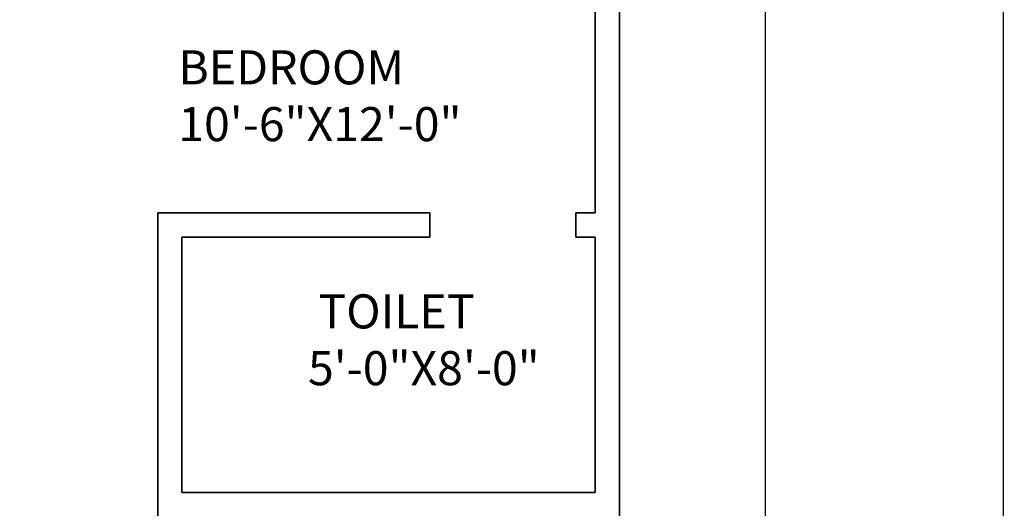
# Model space of a CAD drawing. Units: inches. Extents: x 3731 to 4318, y 1310 to 2388.
# Tile 50 of 57: x 4116 to 4318, y 2129 to 2229. Entities that reach past the tile are written whole.
import ezdxf

# ---------------------------------------------------------------- set-up
doc = ezdxf.new("R2010")
doc.units = ezdxf.units.IN
for name, color, linetype, lineweight in [('A-ANNO-DIMS', 2, 'Continuous', 18), ('A-AREA-IDEN', 7, 'Continuous', 18), ('A-WALL', 7, 'Continuous', 35)]:
    doc.layers.add(name, color=color, linetype=linetype, lineweight=lineweight)
doc.styles.get("Standard").update_dxf_attribs({"font": 'arial.ttf'})
doc.dimstyles.get("Standard").update_dxf_attribs({"dimtxt": 0.18, "dimasz": 0.18, "dimexe": 0.18, "dimexo": 0.0625, "dimgap": 0.09, "dimtad": 0, "dimtih": 1, "dimtoh": 1, "dimdec": 4, "dimzin": 0, "dimdsep": 46, "dimtxsty": 'Standard', "dimcen": 0.09, "dimadec": 0, "dimazin": 0, "dimtfac": 1, "dimtdec": 4, "dimtofl": 0, "dimtmove": 0, "dimatfit": 3, "dimfxl": 1, "dimtolj": 1, "dimtzin": 0, "dimarcsym": 0})

# ---------------------------------------------------------------- blocks, each defined once
blk = doc.blocks.new('*D38')
at = {"layer": 'A-ANNO-DIMS', "color": 0, "lineweight": -2, "transparency": 16777216}
for p, q in [((4103.27, 2262.38), (4318.34, 2262.38)), ((4318.16, 2262.2), (4318.16, 2103.06)), ((4318.16, 1943.56), (4318.16, 2102.7)), ((4234.27, 1943.38), (4318.34, 1943.38))]:
    blk.add_line(p, q, dxfattribs=at)
at = {"layer": 'A-ANNO-DIMS', "color": 0, "transparency": 16777216}
for points in [[(4318.13, 2262.2), (4318.19, 2262.2), (4318.16, 2262.38)], [(4318.13, 1943.56), (4318.19, 1943.56), (4318.16, 1943.38)]]:
    blk.add_solid(points, dxfattribs=at)
at = {"layer": 'Defpoints', "color": 0, "transparency": 16777216}
for p in [(4103.21, 2262.38), (4318.16, 2262.38), (4234.21, 1943.38)]:
    blk.add_point(p, dxfattribs=at)
at = {"layer": 'A-ANNO-DIMS', "color": 0, "transparency": 16777216, "insert": (4318.16, 2102.88), "char_height": 0.18, "attachment_point": 5}
blk.add_mtext('\\A1;319', dxfattribs=at)
blk = doc.blocks.new('*D51')
at = {"layer": 'A-ANNO-DIMS', "color": 0, "lineweight": -2, "transparency": 16777216}
for p, q in [((4239.21, 1708.44), (4239.21, 2387.51)), ((4239.39, 2387.33), (4253.99, 2387.33)), ((4269.03, 2387.33), (4254.43, 2387.33)), ((4269.21, 1708.44), (4269.21, 2387.51))]:
    blk.add_line(p, q, dxfattribs=at)
at = {"layer": 'A-ANNO-DIMS', "color": 0, "transparency": 16777216}
for points in [[(4239.39, 2387.36), (4239.39, 2387.3), (4239.21, 2387.33)], [(4269.03, 2387.36), (4269.03, 2387.3), (4269.21, 2387.33)]]:
    blk.add_solid(points, dxfattribs=at)
at = {"layer": 'Defpoints', "color": 0, "transparency": 16777216}
for p in [(4269.21, 2387.33), (4239.21, 1708.38), (4269.21, 1708.38)]:
    blk.add_point(p, dxfattribs=at)
at = {"layer": 'A-ANNO-DIMS', "color": 0, "transparency": 16777216, "insert": (4254.21, 2387.33), "char_height": 0.18, "attachment_point": 5}
blk.add_mtext('\\A1;30', dxfattribs=at)

msp = doc.modelspace()

# ---------------------------------------------------------------- linework, layer by layer
at = {"layer": 'A-WALL'}
for p, q in [((4239.21, 2338.38), (4239.21, 1708.38)), ((4234.21, 2333.38), (4234.21, 2189.38)), ((4144.21, 2189.38), (4200.21, 2189.38)), ((4144.21, 2189.38), (4144.21, 2069.38)), ((4200.21, 2189.38), (4200.21, 2184.38)), ((4230.21, 2189.38), (4230.21, 2184.38)), ((4230.21, 2189.38), (4234.21, 2189.38)), ((4149.21, 2184.38), (4149.21, 2131.88)), ((4149.21, 2184.38), (4200.21, 2184.38)), ((4230.21, 2184.38), (4234.21, 2184.38)), ((4234.21, 2184.38), (4234.21, 2131.88)), ((4234.21, 2131.88), (4149.21, 2131.88))]:
    msp.add_line(p, q, dxfattribs=at)

# ---------------------------------------------------------------- texts
at = {"layer": 'A-AREA-IDEN', "char_height": 7, "attachment_point": 1}
for s, insert in [('BEDROOM\\P10\'-6"X12\'-0"', (4148.45, 2222.75)), (' TOILET\\P5\'-0"X8\'-0"', (4175.13, 2172.6))]:
    msp.add_mtext_dynamic_manual_height_columns(s, width=39.1687, gutter_width=12.5, heights=[0], dxfattribs=dict(at, insert=insert))

# ---------------------------------------------------------------- dimensions: what is measured, and where the dimension line sits
at = {"layer": 'A-ANNO-DIMS'}
dim = msp.add_linear_dim(base=(4269.21, 2387.33), p1=(4239.21, 1708.38), p2=(4269.21, 1708.38), dimstyle='Standard', override={"dimdec": 0, "dimlfac": 1, "dimrnd": 0, "dimzin": 0, "dimdsep": 46, "dimlunit": 2}, dxfattribs=at)
dim.commit()
dim.dimension.update_dxf_attribs({"geometry": '*D51', "text_midpoint": (4254.21, 2387.33)})
dim = msp.add_linear_dim(base=(4318.16, 2262.38), p1=(4234.21, 1943.38), p2=(4103.21, 2262.38), angle=90, dimstyle='Standard', override={"dimdec": 0, "dimlfac": 1, "dimrnd": 0, "dimzin": 0, "dimdsep": 46, "dimlunit": 2}, dxfattribs=at)
dim.commit()
dim.dimension.update_dxf_attribs({"geometry": '*D38', "text_midpoint": (4318.16, 2102.88)})

doc.saveas('drawing.dxf')
